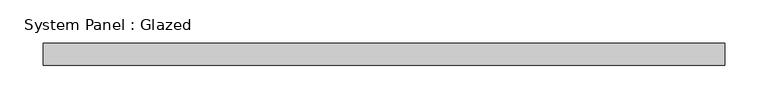
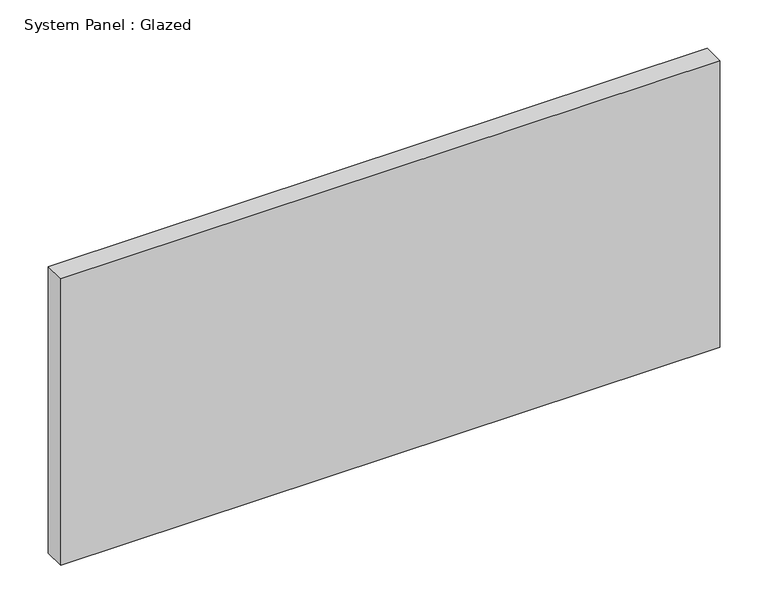
"""IFC4 building model written with IfcOpenShell, lengths in millimetres: plate geometry, System Panel : Glazed."""

from ifc_helpers import new_model, si_unit, origin, origin_with_axes, place, context, project, spatial, polyline, outline, extrude, source, transform, mapped, element, save


def system_panel_glazed_26453c14(model_context):
    return source(origin(), model_context, "Body", "SweptSolid", [
        extrude(outline(polyline([(393.7, 19.05), (-393.7, 19.05), (-393.7, 44.45), (393.7, 44.45), (393.7, 19.05)])), origin_with_axes(), (0.0, 0.0, 1.0), 361.95),
    ])


if __name__ == "__main__":
    model = new_model("IFC4")
    model_context = context("Model", 3, world=origin())
    ifc_project = project(units=[si_unit("LENGTHUNIT", "METRE", prefix="MILLI")], contexts=[model_context])
    site = spatial("IfcSite", under=ifc_project)
    building = spatial("IfcBuilding", under=site)
    placement = place(None, origin())
    system_panel_glazed_shape = system_panel_glazed_26453c14(model_context)
    element("IfcPlate", 1, ObjectType="System Panel : Glazed", at=placement, inside=building, context=model_context, shape_type="MappedRepresentation", body=[
        mapped(system_panel_glazed_shape, transform((0.0, 0.0, 0.0), x_axis=(1.0, 0.0, 0.0), y_axis=(0.0, 1.0, 0.0), z_axis=(0.0, 0.0, 1.0))),
    ])
    save(model, "model.ifc")

# Revit data of these elements
# Type "System Panel : Glazed"
#   Construction Type Id = "GSP4R"
#   Analytic Construction = "1/8 in Pilkington single glazing"
#   Visual Light Transmittance = 0.9
#   Solar Heat Gain Coefficient = 0.86
#   Heat Transfer Coefficient (U) = 1.18115 BTU/(h·ft²·°F)
#   Define Thermal Properties by = 1
# Element 1 (IfcPlate, "System Panel : Glazed")
#   Materials on its faces: "Glass"
# Materials
#   "Glass": class "Glass", colour RGB 0 128 192, transparency 0.75, Description = "Soda Lime Glass", Cost = 0
